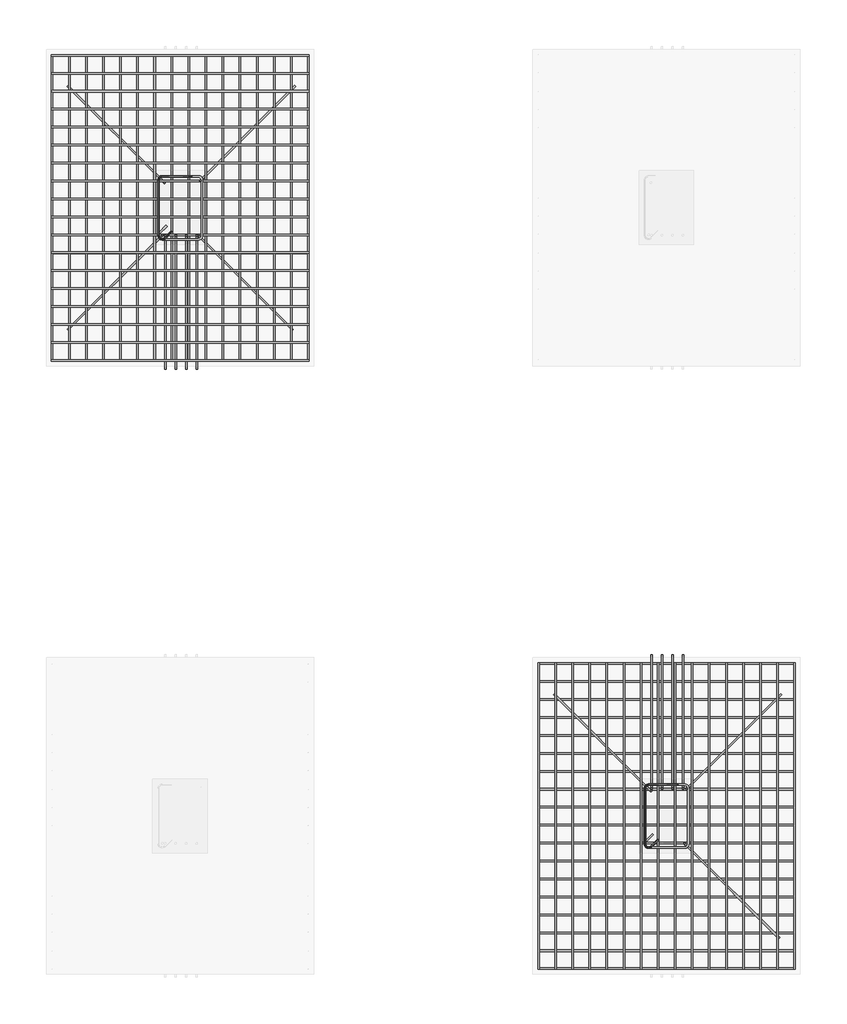
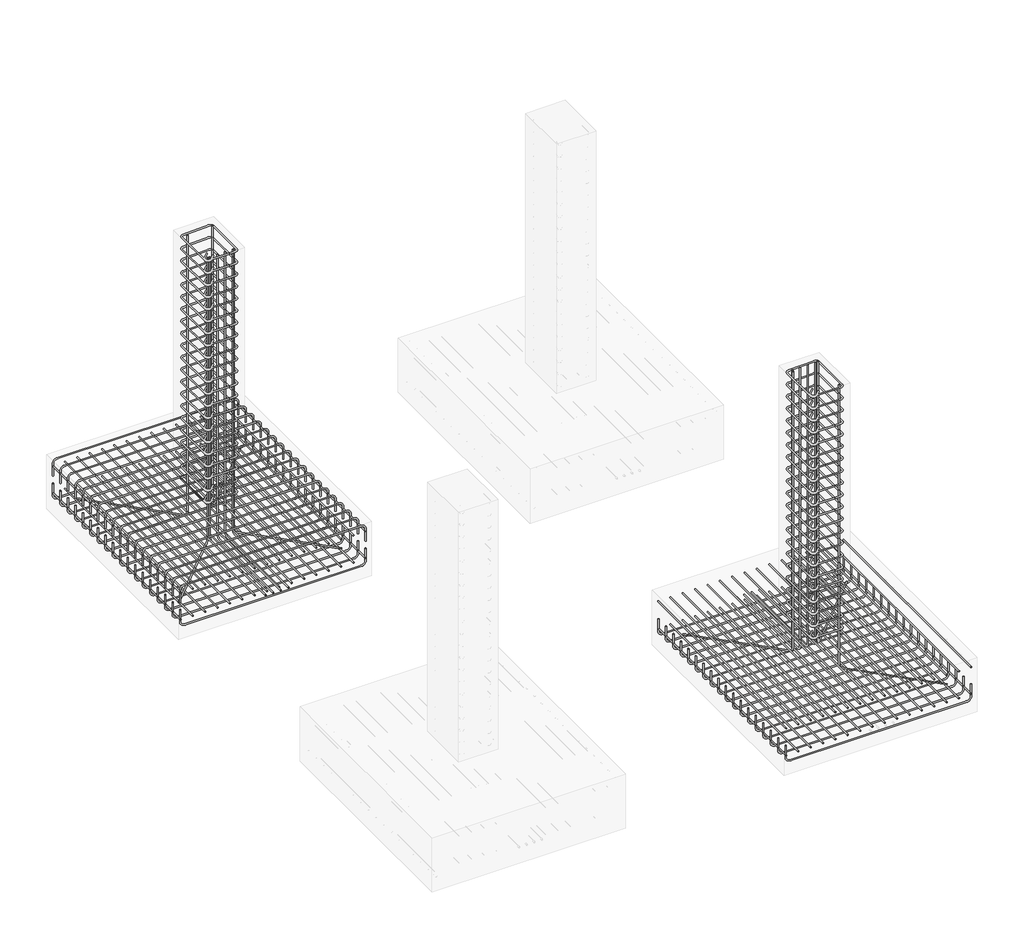
# One storey, part 14 of 33: 18 reinforcing bars.
"""IFC4 building model written with IfcOpenShell, lengths in millimetres."""

from ifc_helpers import new_model, si_unit, point, frame, origin, place, context, project, spatial, polyline, circle_curve, trimmed, segment, composite_curve, source, transform, mapped, element, save
from ifc_brep_helpers import swept_disk

model = new_model("IFC4")

# Units and contexts
model_context = context("Model", 3, world=origin())
ifc_project = project(units=[si_unit("LENGTHUNIT", "METRE", prefix="MILLI")], contexts=[model_context])

# Site, building, storey
site = spatial("IfcSite", under=ifc_project)
building = spatial("IfcBuilding", under=site)
storey = spatial("IfcBuildingStorey", under=building, Elevation=-3000.0)

# Reinforcing bars
placement = place(None, origin())
reinforcing_bar_shape = source(origin(), model_context, "Body", "SolidModel", [
    swept_disk(composite_curve([segment(polyline([(-8586.1642742, 2955.9391866, -3330.080452), (-8586.1642742, 2955.9391866, -3477.380452)]), True, "CONTINUOUS"), segment(trimmed(circle_curve(frame((-8632.5142742, 2955.9391866, -3477.380452), z_axis=(0.0, 1.0, 0.0), x_axis=(46.350000000000364, 0.0, 0.0)), 46.35), [point((-8586.1642742, 2955.9391866, -3477.380452))], [point((-8632.5142742, 2955.9391866, -3523.730452))], True, "CARTESIAN"), True, "CONTINUOUS"), segment(polyline([(-8632.5142742, 2955.9391866, -3523.730452), (-10647.1142742, 2955.9391866, -3523.730452)]), True, "CONTINUOUS"), segment(trimmed(circle_curve(frame((-10647.1142742, 2955.9391866, -3477.380452), z_axis=(0.0, 1.0, 0.0), x_axis=(0.0, 0.0, -46.34999999999991)), 46.35), [point((-10647.1142742, 2955.9391866, -3523.730452))], [point((-10693.4642742, 2955.9391866, -3477.380452))], True, "CARTESIAN"), True, "CONTINUOUS"), segment(polyline([(-10693.4642742, 2955.9391866, -3477.380452), (-10693.4642742, 2955.9391866, -3330.080452)]), True, "CONTINUOUS")], self_intersect=False), 6.35),
])
element("IfcReinforcingBar", 1, at=placement, inside=storey, context=model_context, shape_type="MappedRepresentation", body=[
    mapped(reinforcing_bar_shape, transform((0.0, 0.0, 0.0), x_axis=(1.0, 0.0, 0.0), y_axis=(0.0, 1.0, 0.0), z_axis=(0.0, 0.0, 1.0))),
    mapped(reinforcing_bar_shape, transform((0.0, -147.4882353, 0.0), x_axis=(1.0, 0.0, 0.0), y_axis=(0.0, 1.0, 0.0), z_axis=(0.0, 0.0, 1.0))),
    mapped(reinforcing_bar_shape, transform((0.0, -294.9764706, 0.0), x_axis=(1.0, 0.0, 0.0), y_axis=(0.0, 1.0, 0.0), z_axis=(0.0, 0.0, 1.0))),
    mapped(reinforcing_bar_shape, transform((0.0, -442.4647059, 0.0), x_axis=(1.0, 0.0, 0.0), y_axis=(0.0, 1.0, 0.0), z_axis=(0.0, 0.0, 1.0))),
    mapped(reinforcing_bar_shape, transform((0.0, -589.9529412, 0.0), x_axis=(1.0, 0.0, 0.0), y_axis=(0.0, 1.0, 0.0), z_axis=(0.0, 0.0, 1.0))),
    mapped(reinforcing_bar_shape, transform((0.0, -737.4411765, 0.0), x_axis=(1.0, 0.0, 0.0), y_axis=(0.0, 1.0, 0.0), z_axis=(0.0, 0.0, 1.0))),
    mapped(reinforcing_bar_shape, transform((0.0, -884.9294118, 0.0), x_axis=(1.0, 0.0, 0.0), y_axis=(0.0, 1.0, 0.0), z_axis=(0.0, 0.0, 1.0))),
    mapped(reinforcing_bar_shape, transform((0.0, -1032.4176471, 0.0), x_axis=(1.0, 0.0, 0.0), y_axis=(0.0, 1.0, 0.0), z_axis=(0.0, 0.0, 1.0))),
    mapped(reinforcing_bar_shape, transform((0.0, -1179.9058824, 0.0), x_axis=(1.0, 0.0, 0.0), y_axis=(0.0, 1.0, 0.0), z_axis=(0.0, 0.0, 1.0))),
    mapped(reinforcing_bar_shape, transform((0.0, -1327.3941176, 0.0), x_axis=(1.0, 0.0, 0.0), y_axis=(0.0, 1.0, 0.0), z_axis=(0.0, 0.0, 1.0))),
    mapped(reinforcing_bar_shape, transform((0.0, -1474.8823529, 0.0), x_axis=(1.0, 0.0, 0.0), y_axis=(0.0, 1.0, 0.0), z_axis=(0.0, 0.0, 1.0))),
    mapped(reinforcing_bar_shape, transform((0.0, -1622.3705882, 0.0), x_axis=(1.0, 0.0, 0.0), y_axis=(0.0, 1.0, 0.0), z_axis=(0.0, 0.0, 1.0))),
    mapped(reinforcing_bar_shape, transform((0.0, -1769.8588235, 0.0), x_axis=(1.0, 0.0, 0.0), y_axis=(0.0, 1.0, 0.0), z_axis=(0.0, 0.0, 1.0))),
    mapped(reinforcing_bar_shape, transform((0.0, -1917.3470588, 0.0), x_axis=(1.0, 0.0, 0.0), y_axis=(0.0, 1.0, 0.0), z_axis=(0.0, 0.0, 1.0))),
    mapped(reinforcing_bar_shape, transform((0.0, -2064.8352941, 0.0), x_axis=(1.0, 0.0, 0.0), y_axis=(0.0, 1.0, 0.0), z_axis=(0.0, 0.0, 1.0))),
    mapped(reinforcing_bar_shape, transform((0.0, -2212.3235294, 0.0), x_axis=(1.0, 0.0, 0.0), y_axis=(0.0, 1.0, 0.0), z_axis=(0.0, 0.0, 1.0))),
    mapped(reinforcing_bar_shape, transform((0.0, -2359.8117647, 0.0), x_axis=(1.0, 0.0, 0.0), y_axis=(0.0, 1.0, 0.0), z_axis=(0.0, 0.0, 1.0))),
    mapped(reinforcing_bar_shape, transform((0.0, -2507.3, 0.0), x_axis=(1.0, 0.0, 0.0), y_axis=(0.0, 1.0, 0.0), z_axis=(0.0, 0.0, 1.0))),
])
reinforcing_bar_2_shape = source(origin(), model_context, "Body", "SolidModel", [
    swept_disk(composite_curve([segment(polyline([(-8586.1642742, 442.2891866, -3447.8614173), (-8586.1642742, 2962.2891866, -3447.8614173)]), True, "CONTINUOUS")], self_intersect=False), 6.35),
])
element("IfcReinforcingBar", 2, at=placement, inside=storey, context=model_context, shape_type="MappedRepresentation", body=[
    mapped(reinforcing_bar_2_shape, transform((0.0, 0.0, 0.0), x_axis=(1.0, 0.0, 0.0), y_axis=(0.0, 1.0, 0.0), z_axis=(0.0, 0.0, 1.0))),
    mapped(reinforcing_bar_2_shape, transform((-140.4866667, 0.0, 0.0), x_axis=(1.0, 0.0, 0.0), y_axis=(0.0, 1.0, 0.0), z_axis=(0.0, 0.0, 1.0))),
    mapped(reinforcing_bar_2_shape, transform((-280.9733333, 0.0, 0.0), x_axis=(1.0, 0.0, 0.0), y_axis=(0.0, 1.0, 0.0), z_axis=(0.0, 0.0, 1.0))),
    mapped(reinforcing_bar_2_shape, transform((-421.46, 0.0, 0.0), x_axis=(1.0, 0.0, 0.0), y_axis=(0.0, 1.0, 0.0), z_axis=(0.0, 0.0, 1.0))),
    mapped(reinforcing_bar_2_shape, transform((-561.9466667, 0.0, 0.0), x_axis=(1.0, 0.0, 0.0), y_axis=(0.0, 1.0, 0.0), z_axis=(0.0, 0.0, 1.0))),
    mapped(reinforcing_bar_2_shape, transform((-702.4333333, 0.0, 0.0), x_axis=(1.0, 0.0, 0.0), y_axis=(0.0, 1.0, 0.0), z_axis=(0.0, 0.0, 1.0))),
    mapped(reinforcing_bar_2_shape, transform((-842.92, 0.0, 0.0), x_axis=(1.0, 0.0, 0.0), y_axis=(0.0, 1.0, 0.0), z_axis=(0.0, 0.0, 1.0))),
    mapped(reinforcing_bar_2_shape, transform((-983.4066667, 0.0, 0.0), x_axis=(1.0, 0.0, 0.0), y_axis=(0.0, 1.0, 0.0), z_axis=(0.0, 0.0, 1.0))),
    mapped(reinforcing_bar_2_shape, transform((-1123.8933333, 0.0, 0.0), x_axis=(1.0, 0.0, 0.0), y_axis=(0.0, 1.0, 0.0), z_axis=(0.0, 0.0, 1.0))),
    mapped(reinforcing_bar_2_shape, transform((-1264.38, 0.0, 0.0), x_axis=(1.0, 0.0, 0.0), y_axis=(0.0, 1.0, 0.0), z_axis=(0.0, 0.0, 1.0))),
    mapped(reinforcing_bar_2_shape, transform((-1404.8666667, 0.0, 0.0), x_axis=(1.0, 0.0, 0.0), y_axis=(0.0, 1.0, 0.0), z_axis=(0.0, 0.0, 1.0))),
    mapped(reinforcing_bar_2_shape, transform((-1545.3533333, 0.0, 0.0), x_axis=(1.0, 0.0, 0.0), y_axis=(0.0, 1.0, 0.0), z_axis=(0.0, 0.0, 1.0))),
    mapped(reinforcing_bar_2_shape, transform((-1685.84, 0.0, 0.0), x_axis=(1.0, 0.0, 0.0), y_axis=(0.0, 1.0, 0.0), z_axis=(0.0, 0.0, 1.0))),
    mapped(reinforcing_bar_2_shape, transform((-1826.3266667, 0.0, 0.0), x_axis=(1.0, 0.0, 0.0), y_axis=(0.0, 1.0, 0.0), z_axis=(0.0, 0.0, 1.0))),
    mapped(reinforcing_bar_2_shape, transform((-1966.8133333, 0.0, 0.0), x_axis=(1.0, 0.0, 0.0), y_axis=(0.0, 1.0, 0.0), z_axis=(0.0, 0.0, 1.0))),
    mapped(reinforcing_bar_2_shape, transform((-2107.3, 0.0, 0.0), x_axis=(1.0, 0.0, 0.0), y_axis=(0.0, 1.0, 0.0), z_axis=(0.0, 0.0, 1.0))),
])
reinforcing_bar_3_shape = source(origin(), model_context, "Body", "SolidModel", [
    swept_disk(composite_curve([segment(polyline([(-10693.4642742, 442.2891866, -3122.7084113), (-10693.4642742, 2962.2891866, -3122.7084113)]), True, "CONTINUOUS")], self_intersect=False), 6.35),
])
element("IfcReinforcingBar", 3, at=placement, inside=storey, context=model_context, shape_type="MappedRepresentation", body=[
    mapped(reinforcing_bar_3_shape, transform((0.0, 0.0, 0.0), x_axis=(1.0, 0.0, 0.0), y_axis=(0.0, 1.0, 0.0), z_axis=(0.0, 0.0, 1.0))),
    mapped(reinforcing_bar_3_shape, transform((140.4866667, 0.0, 0.0), x_axis=(1.0, 0.0, 0.0), y_axis=(0.0, 1.0, 0.0), z_axis=(0.0, 0.0, 1.0))),
    mapped(reinforcing_bar_3_shape, transform((280.9733333, 0.0, 0.0), x_axis=(1.0, 0.0, 0.0), y_axis=(0.0, 1.0, 0.0), z_axis=(0.0, 0.0, 1.0))),
    mapped(reinforcing_bar_3_shape, transform((421.46, 0.0, 0.0), x_axis=(1.0, 0.0, 0.0), y_axis=(0.0, 1.0, 0.0), z_axis=(0.0, 0.0, 1.0))),
    mapped(reinforcing_bar_3_shape, transform((561.9466667, 0.0, 0.0), x_axis=(1.0, 0.0, 0.0), y_axis=(0.0, 1.0, 0.0), z_axis=(0.0, 0.0, 1.0))),
    mapped(reinforcing_bar_3_shape, transform((702.4333333, 0.0, 0.0), x_axis=(1.0, 0.0, 0.0), y_axis=(0.0, 1.0, 0.0), z_axis=(0.0, 0.0, 1.0))),
    mapped(reinforcing_bar_3_shape, transform((842.92, 0.0, 0.0), x_axis=(1.0, 0.0, 0.0), y_axis=(0.0, 1.0, 0.0), z_axis=(0.0, 0.0, 1.0))),
    mapped(reinforcing_bar_3_shape, transform((983.4066667, 0.0, 0.0), x_axis=(1.0, 0.0, 0.0), y_axis=(0.0, 1.0, 0.0), z_axis=(0.0, 0.0, 1.0))),
    mapped(reinforcing_bar_3_shape, transform((1123.8933333, 0.0, 0.0), x_axis=(1.0, 0.0, 0.0), y_axis=(0.0, 1.0, 0.0), z_axis=(0.0, 0.0, 1.0))),
    mapped(reinforcing_bar_3_shape, transform((1264.38, 0.0, 0.0), x_axis=(1.0, 0.0, 0.0), y_axis=(0.0, 1.0, 0.0), z_axis=(0.0, 0.0, 1.0))),
    mapped(reinforcing_bar_3_shape, transform((1404.8666667, 0.0, 0.0), x_axis=(1.0, 0.0, 0.0), y_axis=(0.0, 1.0, 0.0), z_axis=(0.0, 0.0, 1.0))),
    mapped(reinforcing_bar_3_shape, transform((1545.3533333, 0.0, 0.0), x_axis=(1.0, 0.0, 0.0), y_axis=(0.0, 1.0, 0.0), z_axis=(0.0, 0.0, 1.0))),
    mapped(reinforcing_bar_3_shape, transform((1685.84, 0.0, 0.0), x_axis=(1.0, 0.0, 0.0), y_axis=(0.0, 1.0, 0.0), z_axis=(0.0, 0.0, 1.0))),
    mapped(reinforcing_bar_3_shape, transform((1826.3266667, 0.0, 0.0), x_axis=(1.0, 0.0, 0.0), y_axis=(0.0, 1.0, 0.0), z_axis=(0.0, 0.0, 1.0))),
    mapped(reinforcing_bar_3_shape, transform((1966.8133333, 0.0, 0.0), x_axis=(1.0, 0.0, 0.0), y_axis=(0.0, 1.0, 0.0), z_axis=(0.0, 0.0, 1.0))),
    mapped(reinforcing_bar_3_shape, transform((2107.3, 0.0, 0.0), x_axis=(1.0, 0.0, 0.0), y_axis=(0.0, 1.0, 0.0), z_axis=(0.0, 0.0, 1.0))),
])
reinforcing_bar_4_shape = source(origin(), model_context, "Body", "SolidModel", [
    swept_disk(composite_curve([segment(polyline([(-14693.4642742, 7955.9391866, -3240.0), (-14693.4642742, 7955.9391866, -3092.7)]), True, "CONTINUOUS"), segment(trimmed(circle_curve(frame((-14647.1142742, 7955.9391866, -3092.7), z_axis=(0.0, 1.0, 0.0), x_axis=(-46.350000000000364, 0.0, 0.0)), 46.35), [point((-14693.4642742, 7955.9391866, -3092.7))], [point((-14647.1142742, 7955.9391866, -3046.35))], True, "CARTESIAN"), True, "CONTINUOUS"), segment(polyline([(-14647.1142742, 7955.9391866, -3046.35), (-12632.5142742, 7955.9391866, -3046.35)]), True, "CONTINUOUS"), segment(trimmed(circle_curve(frame((-12632.5142742, 7955.9391866, -3092.7), z_axis=(0.0, 1.0, 0.0), x_axis=(0.0, 0.0, 46.34999999999991)), 46.35), [point((-12632.5142742, 7955.9391866, -3046.35))], [point((-12586.1642742, 7955.9391866, -3092.7))], True, "CARTESIAN"), True, "CONTINUOUS"), segment(polyline([(-12586.1642742, 7955.9391866, -3092.7), (-12586.1642742, 7955.9391866, -3240.0)]), True, "CONTINUOUS")], self_intersect=False), 6.35),
])
element("IfcReinforcingBar", 4, at=placement, inside=storey, context=model_context, shape_type="MappedRepresentation", body=[
    mapped(reinforcing_bar_4_shape, transform((0.0, 0.0, 0.0), x_axis=(1.0, 0.0, 0.0), y_axis=(0.0, 1.0, 0.0), z_axis=(0.0, 0.0, 1.0))),
    mapped(reinforcing_bar_4_shape, transform((0.0, -147.4882353, 0.0), x_axis=(1.0, 0.0, 0.0), y_axis=(0.0, 1.0, 0.0), z_axis=(0.0, 0.0, 1.0))),
    mapped(reinforcing_bar_4_shape, transform((0.0, -294.9764706, 0.0), x_axis=(1.0, 0.0, 0.0), y_axis=(0.0, 1.0, 0.0), z_axis=(0.0, 0.0, 1.0))),
    mapped(reinforcing_bar_4_shape, transform((0.0, -442.4647059, 0.0), x_axis=(1.0, 0.0, 0.0), y_axis=(0.0, 1.0, 0.0), z_axis=(0.0, 0.0, 1.0))),
    mapped(reinforcing_bar_4_shape, transform((0.0, -589.9529412, 0.0), x_axis=(1.0, 0.0, 0.0), y_axis=(0.0, 1.0, 0.0), z_axis=(0.0, 0.0, 1.0))),
    mapped(reinforcing_bar_4_shape, transform((0.0, -737.4411765, 0.0), x_axis=(1.0, 0.0, 0.0), y_axis=(0.0, 1.0, 0.0), z_axis=(0.0, 0.0, 1.0))),
    mapped(reinforcing_bar_4_shape, transform((0.0, -884.9294118, 0.0), x_axis=(1.0, 0.0, 0.0), y_axis=(0.0, 1.0, 0.0), z_axis=(0.0, 0.0, 1.0))),
    mapped(reinforcing_bar_4_shape, transform((0.0, -1032.4176471, 0.0), x_axis=(1.0, 0.0, 0.0), y_axis=(0.0, 1.0, 0.0), z_axis=(0.0, 0.0, 1.0))),
    mapped(reinforcing_bar_4_shape, transform((0.0, -1179.9058824, 0.0), x_axis=(1.0, 0.0, 0.0), y_axis=(0.0, 1.0, 0.0), z_axis=(0.0, 0.0, 1.0))),
    mapped(reinforcing_bar_4_shape, transform((0.0, -1327.3941176, 0.0), x_axis=(1.0, 0.0, 0.0), y_axis=(0.0, 1.0, 0.0), z_axis=(0.0, 0.0, 1.0))),
    mapped(reinforcing_bar_4_shape, transform((0.0, -1474.8823529, 0.0), x_axis=(1.0, 0.0, 0.0), y_axis=(0.0, 1.0, 0.0), z_axis=(0.0, 0.0, 1.0))),
    mapped(reinforcing_bar_4_shape, transform((0.0, -1622.3705882, 0.0), x_axis=(1.0, 0.0, 0.0), y_axis=(0.0, 1.0, 0.0), z_axis=(0.0, 0.0, 1.0))),
    mapped(reinforcing_bar_4_shape, transform((0.0, -1769.8588235, 0.0), x_axis=(1.0, 0.0, 0.0), y_axis=(0.0, 1.0, 0.0), z_axis=(0.0, 0.0, 1.0))),
    mapped(reinforcing_bar_4_shape, transform((0.0, -1917.3470588, 0.0), x_axis=(1.0, 0.0, 0.0), y_axis=(0.0, 1.0, 0.0), z_axis=(0.0, 0.0, 1.0))),
    mapped(reinforcing_bar_4_shape, transform((0.0, -2064.8352941, 0.0), x_axis=(1.0, 0.0, 0.0), y_axis=(0.0, 1.0, 0.0), z_axis=(0.0, 0.0, 1.0))),
    mapped(reinforcing_bar_4_shape, transform((0.0, -2212.3235294, 0.0), x_axis=(1.0, 0.0, 0.0), y_axis=(0.0, 1.0, 0.0), z_axis=(0.0, 0.0, 1.0))),
    mapped(reinforcing_bar_4_shape, transform((0.0, -2359.8117647, 0.0), x_axis=(1.0, 0.0, 0.0), y_axis=(0.0, 1.0, 0.0), z_axis=(0.0, 0.0, 1.0))),
    mapped(reinforcing_bar_4_shape, transform((0.0, -2507.3, 0.0), x_axis=(1.0, 0.0, 0.0), y_axis=(0.0, 1.0, 0.0), z_axis=(0.0, 0.0, 1.0))),
])
reinforcing_bar_5_shape = source(origin(), model_context, "Body", "SolidModel", [
    swept_disk(composite_curve([segment(polyline([(-12586.1642742, 7955.9391866, -3330.080452), (-12586.1642742, 7955.9391866, -3477.380452)]), True, "CONTINUOUS"), segment(trimmed(circle_curve(frame((-12632.5142742, 7955.9391866, -3477.380452), z_axis=(0.0, 1.0, 0.0), x_axis=(46.350000000000364, 0.0, 0.0)), 46.35), [point((-12586.1642742, 7955.9391866, -3477.380452))], [point((-12632.5142742, 7955.9391866, -3523.730452))], True, "CARTESIAN"), True, "CONTINUOUS"), segment(polyline([(-12632.5142742, 7955.9391866, -3523.730452), (-14647.1142742, 7955.9391866, -3523.730452)]), True, "CONTINUOUS"), segment(trimmed(circle_curve(frame((-14647.1142742, 7955.9391866, -3477.380452), z_axis=(0.0, 1.0, 0.0), x_axis=(0.0, 0.0, -46.34999999999991)), 46.35), [point((-14647.1142742, 7955.9391866, -3523.730452))], [point((-14693.4642742, 7955.9391866, -3477.380452))], True, "CARTESIAN"), True, "CONTINUOUS"), segment(polyline([(-14693.4642742, 7955.9391866, -3477.380452), (-14693.4642742, 7955.9391866, -3330.080452)]), True, "CONTINUOUS")], self_intersect=False), 6.35),
])
element("IfcReinforcingBar", 5, at=placement, inside=storey, context=model_context, shape_type="MappedRepresentation", body=[
    mapped(reinforcing_bar_5_shape, transform((0.0, 0.0, 0.0), x_axis=(1.0, 0.0, 0.0), y_axis=(0.0, 1.0, 0.0), z_axis=(0.0, 0.0, 1.0))),
    mapped(reinforcing_bar_5_shape, transform((0.0, -147.4882353, 0.0), x_axis=(1.0, 0.0, 0.0), y_axis=(0.0, 1.0, 0.0), z_axis=(0.0, 0.0, 1.0))),
    mapped(reinforcing_bar_5_shape, transform((0.0, -294.9764706, 0.0), x_axis=(1.0, 0.0, 0.0), y_axis=(0.0, 1.0, 0.0), z_axis=(0.0, 0.0, 1.0))),
    mapped(reinforcing_bar_5_shape, transform((0.0, -442.4647059, 0.0), x_axis=(1.0, 0.0, 0.0), y_axis=(0.0, 1.0, 0.0), z_axis=(0.0, 0.0, 1.0))),
    mapped(reinforcing_bar_5_shape, transform((0.0, -589.9529412, 0.0), x_axis=(1.0, 0.0, 0.0), y_axis=(0.0, 1.0, 0.0), z_axis=(0.0, 0.0, 1.0))),
    mapped(reinforcing_bar_5_shape, transform((0.0, -737.4411765, 0.0), x_axis=(1.0, 0.0, 0.0), y_axis=(0.0, 1.0, 0.0), z_axis=(0.0, 0.0, 1.0))),
    mapped(reinforcing_bar_5_shape, transform((0.0, -884.9294118, 0.0), x_axis=(1.0, 0.0, 0.0), y_axis=(0.0, 1.0, 0.0), z_axis=(0.0, 0.0, 1.0))),
    mapped(reinforcing_bar_5_shape, transform((0.0, -1032.4176471, 0.0), x_axis=(1.0, 0.0, 0.0), y_axis=(0.0, 1.0, 0.0), z_axis=(0.0, 0.0, 1.0))),
    mapped(reinforcing_bar_5_shape, transform((0.0, -1179.9058824, 0.0), x_axis=(1.0, 0.0, 0.0), y_axis=(0.0, 1.0, 0.0), z_axis=(0.0, 0.0, 1.0))),
    mapped(reinforcing_bar_5_shape, transform((0.0, -1327.3941176, 0.0), x_axis=(1.0, 0.0, 0.0), y_axis=(0.0, 1.0, 0.0), z_axis=(0.0, 0.0, 1.0))),
    mapped(reinforcing_bar_5_shape, transform((0.0, -1474.8823529, 0.0), x_axis=(1.0, 0.0, 0.0), y_axis=(0.0, 1.0, 0.0), z_axis=(0.0, 0.0, 1.0))),
    mapped(reinforcing_bar_5_shape, transform((0.0, -1622.3705882, 0.0), x_axis=(1.0, 0.0, 0.0), y_axis=(0.0, 1.0, 0.0), z_axis=(0.0, 0.0, 1.0))),
    mapped(reinforcing_bar_5_shape, transform((0.0, -1769.8588235, 0.0), x_axis=(1.0, 0.0, 0.0), y_axis=(0.0, 1.0, 0.0), z_axis=(0.0, 0.0, 1.0))),
    mapped(reinforcing_bar_5_shape, transform((0.0, -1917.3470588, 0.0), x_axis=(1.0, 0.0, 0.0), y_axis=(0.0, 1.0, 0.0), z_axis=(0.0, 0.0, 1.0))),
    mapped(reinforcing_bar_5_shape, transform((0.0, -2064.8352941, 0.0), x_axis=(1.0, 0.0, 0.0), y_axis=(0.0, 1.0, 0.0), z_axis=(0.0, 0.0, 1.0))),
    mapped(reinforcing_bar_5_shape, transform((0.0, -2212.3235294, 0.0), x_axis=(1.0, 0.0, 0.0), y_axis=(0.0, 1.0, 0.0), z_axis=(0.0, 0.0, 1.0))),
    mapped(reinforcing_bar_5_shape, transform((0.0, -2359.8117647, 0.0), x_axis=(1.0, 0.0, 0.0), y_axis=(0.0, 1.0, 0.0), z_axis=(0.0, 0.0, 1.0))),
    mapped(reinforcing_bar_5_shape, transform((0.0, -2507.3, 0.0), x_axis=(1.0, 0.0, 0.0), y_axis=(0.0, 1.0, 0.0), z_axis=(0.0, 0.0, 1.0))),
])
reinforcing_bar_6_shape = source(origin(), model_context, "Body", "SolidModel", [
    swept_disk(composite_curve([segment(polyline([(-12586.1642742, 5442.2891866, -3447.8614173), (-12586.1642742, 7962.2891866, -3447.8614173)]), True, "CONTINUOUS")], self_intersect=False), 6.35),
])
element("IfcReinforcingBar", 6, at=placement, inside=storey, context=model_context, shape_type="MappedRepresentation", body=[
    mapped(reinforcing_bar_6_shape, transform((0.0, 0.0, 0.0), x_axis=(1.0, 0.0, 0.0), y_axis=(0.0, 1.0, 0.0), z_axis=(0.0, 0.0, 1.0))),
    mapped(reinforcing_bar_6_shape, transform((-140.4866667, 0.0, 0.0), x_axis=(1.0, 0.0, 0.0), y_axis=(0.0, 1.0, 0.0), z_axis=(0.0, 0.0, 1.0))),
    mapped(reinforcing_bar_6_shape, transform((-280.9733333, 0.0, 0.0), x_axis=(1.0, 0.0, 0.0), y_axis=(0.0, 1.0, 0.0), z_axis=(0.0, 0.0, 1.0))),
    mapped(reinforcing_bar_6_shape, transform((-421.46, 0.0, 0.0), x_axis=(1.0, 0.0, 0.0), y_axis=(0.0, 1.0, 0.0), z_axis=(0.0, 0.0, 1.0))),
    mapped(reinforcing_bar_6_shape, transform((-561.9466667, 0.0, 0.0), x_axis=(1.0, 0.0, 0.0), y_axis=(0.0, 1.0, 0.0), z_axis=(0.0, 0.0, 1.0))),
    mapped(reinforcing_bar_6_shape, transform((-702.4333333, 0.0, 0.0), x_axis=(1.0, 0.0, 0.0), y_axis=(0.0, 1.0, 0.0), z_axis=(0.0, 0.0, 1.0))),
    mapped(reinforcing_bar_6_shape, transform((-842.92, 0.0, 0.0), x_axis=(1.0, 0.0, 0.0), y_axis=(0.0, 1.0, 0.0), z_axis=(0.0, 0.0, 1.0))),
    mapped(reinforcing_bar_6_shape, transform((-983.4066667, 0.0, 0.0), x_axis=(1.0, 0.0, 0.0), y_axis=(0.0, 1.0, 0.0), z_axis=(0.0, 0.0, 1.0))),
    mapped(reinforcing_bar_6_shape, transform((-1123.8933333, 0.0, 0.0), x_axis=(1.0, 0.0, 0.0), y_axis=(0.0, 1.0, 0.0), z_axis=(0.0, 0.0, 1.0))),
    mapped(reinforcing_bar_6_shape, transform((-1264.38, 0.0, 0.0), x_axis=(1.0, 0.0, 0.0), y_axis=(0.0, 1.0, 0.0), z_axis=(0.0, 0.0, 1.0))),
    mapped(reinforcing_bar_6_shape, transform((-1404.8666667, 0.0, 0.0), x_axis=(1.0, 0.0, 0.0), y_axis=(0.0, 1.0, 0.0), z_axis=(0.0, 0.0, 1.0))),
    mapped(reinforcing_bar_6_shape, transform((-1545.3533333, 0.0, 0.0), x_axis=(1.0, 0.0, 0.0), y_axis=(0.0, 1.0, 0.0), z_axis=(0.0, 0.0, 1.0))),
    mapped(reinforcing_bar_6_shape, transform((-1685.84, 0.0, 0.0), x_axis=(1.0, 0.0, 0.0), y_axis=(0.0, 1.0, 0.0), z_axis=(0.0, 0.0, 1.0))),
    mapped(reinforcing_bar_6_shape, transform((-1826.3266667, 0.0, 0.0), x_axis=(1.0, 0.0, 0.0), y_axis=(0.0, 1.0, 0.0), z_axis=(0.0, 0.0, 1.0))),
    mapped(reinforcing_bar_6_shape, transform((-1966.8133333, 0.0, 0.0), x_axis=(1.0, 0.0, 0.0), y_axis=(0.0, 1.0, 0.0), z_axis=(0.0, 0.0, 1.0))),
    mapped(reinforcing_bar_6_shape, transform((-2107.3, 0.0, 0.0), x_axis=(1.0, 0.0, 0.0), y_axis=(0.0, 1.0, 0.0), z_axis=(0.0, 0.0, 1.0))),
])
reinforcing_bar_7_shape = source(origin(), model_context, "Body", "SolidModel", [
    swept_disk(composite_curve([segment(polyline([(-14693.4642742, 5442.2891866, -3122.7084113), (-14693.4642742, 7962.2891866, -3122.7084113)]), True, "CONTINUOUS")], self_intersect=False), 6.35),
])
element("IfcReinforcingBar", 7, at=placement, inside=storey, context=model_context, shape_type="MappedRepresentation", body=[
    mapped(reinforcing_bar_7_shape, transform((0.0, 0.0, 0.0), x_axis=(1.0, 0.0, 0.0), y_axis=(0.0, 1.0, 0.0), z_axis=(0.0, 0.0, 1.0))),
    mapped(reinforcing_bar_7_shape, transform((140.4866667, 0.0, 0.0), x_axis=(1.0, 0.0, 0.0), y_axis=(0.0, 1.0, 0.0), z_axis=(0.0, 0.0, 1.0))),
    mapped(reinforcing_bar_7_shape, transform((280.9733333, 0.0, 0.0), x_axis=(1.0, 0.0, 0.0), y_axis=(0.0, 1.0, 0.0), z_axis=(0.0, 0.0, 1.0))),
    mapped(reinforcing_bar_7_shape, transform((421.46, 0.0, 0.0), x_axis=(1.0, 0.0, 0.0), y_axis=(0.0, 1.0, 0.0), z_axis=(0.0, 0.0, 1.0))),
    mapped(reinforcing_bar_7_shape, transform((561.9466667, 0.0, 0.0), x_axis=(1.0, 0.0, 0.0), y_axis=(0.0, 1.0, 0.0), z_axis=(0.0, 0.0, 1.0))),
    mapped(reinforcing_bar_7_shape, transform((702.4333333, 0.0, 0.0), x_axis=(1.0, 0.0, 0.0), y_axis=(0.0, 1.0, 0.0), z_axis=(0.0, 0.0, 1.0))),
    mapped(reinforcing_bar_7_shape, transform((842.92, 0.0, 0.0), x_axis=(1.0, 0.0, 0.0), y_axis=(0.0, 1.0, 0.0), z_axis=(0.0, 0.0, 1.0))),
    mapped(reinforcing_bar_7_shape, transform((983.4066667, 0.0, 0.0), x_axis=(1.0, 0.0, 0.0), y_axis=(0.0, 1.0, 0.0), z_axis=(0.0, 0.0, 1.0))),
    mapped(reinforcing_bar_7_shape, transform((1123.8933333, 0.0, 0.0), x_axis=(1.0, 0.0, 0.0), y_axis=(0.0, 1.0, 0.0), z_axis=(0.0, 0.0, 1.0))),
    mapped(reinforcing_bar_7_shape, transform((1264.38, 0.0, 0.0), x_axis=(1.0, 0.0, 0.0), y_axis=(0.0, 1.0, 0.0), z_axis=(0.0, 0.0, 1.0))),
    mapped(reinforcing_bar_7_shape, transform((1404.8666667, 0.0, 0.0), x_axis=(1.0, 0.0, 0.0), y_axis=(0.0, 1.0, 0.0), z_axis=(0.0, 0.0, 1.0))),
    mapped(reinforcing_bar_7_shape, transform((1545.3533333, 0.0, 0.0), x_axis=(1.0, 0.0, 0.0), y_axis=(0.0, 1.0, 0.0), z_axis=(0.0, 0.0, 1.0))),
    mapped(reinforcing_bar_7_shape, transform((1685.84, 0.0, 0.0), x_axis=(1.0, 0.0, 0.0), y_axis=(0.0, 1.0, 0.0), z_axis=(0.0, 0.0, 1.0))),
    mapped(reinforcing_bar_7_shape, transform((1826.3266667, 0.0, 0.0), x_axis=(1.0, 0.0, 0.0), y_axis=(0.0, 1.0, 0.0), z_axis=(0.0, 0.0, 1.0))),
    mapped(reinforcing_bar_7_shape, transform((1966.8133333, 0.0, 0.0), x_axis=(1.0, 0.0, 0.0), y_axis=(0.0, 1.0, 0.0), z_axis=(0.0, 0.0, 1.0))),
    mapped(reinforcing_bar_7_shape, transform((2107.3, 0.0, 0.0), x_axis=(1.0, 0.0, 0.0), y_axis=(0.0, 1.0, 0.0), z_axis=(0.0, 0.0, 1.0))),
])
reinforcing_bar_8_shape = source(origin(), model_context, "Body", "SolidModel", [
    swept_disk(composite_curve([segment(polyline([(-13753.5385089, 6553.1005472, -2953.65), (-13809.2820718, 6497.3569842, -2953.65)]), True, "CONTINUOUS"), segment(trimmed(circle_curve(frame((-13787.1142742, 6475.1891866, -2953.65), z_axis=(0.0, 0.0, 1.0), x_axis=(-22.167797600000995, 22.167797600000085, 0.0)), 31.35), [point((-13809.2820718, 6497.3569842, -2953.65))], [point((-13787.1142742, 6443.8391866, -2953.65))], True, "CARTESIAN"), True, "CONTINUOUS"), segment(polyline([(-13787.1142742, 6443.8391866, -2953.65), (-13492.5142742, 6443.8391866, -2953.65)]), True, "CONTINUOUS"), segment(trimmed(circle_curve(frame((-13492.5142742, 6475.1891866, -2953.65), z_axis=(0.0, 0.0, 1.0), x_axis=(0.0, -31.349999999999454, 0.0)), 31.35), [point((-13492.5142742, 6443.8391866, -2953.65))], [point((-13461.1642742, 6475.1891866, -2953.65))], True, "CARTESIAN"), True, "CONTINUOUS"), segment(polyline([(-13461.1642742, 6475.1891866, -2953.65), (-13461.1642742, 6929.3891866, -2953.65)]), True, "CONTINUOUS"), segment(trimmed(circle_curve(frame((-13492.4944891, 6929.3891866, -2954.7636125), z_axis=(-0.0355219283344822, 0.0, 0.9993688971583016), x_axis=(31.33021489999919, 0.0, 1.1136124999998174)), 31.35), [point((-13461.1642742, 6929.3891866, -2953.65))], [point((-13492.4944891, 6960.7391866, -2954.7636125))], True, "CARTESIAN"), True, "CONTINUOUS"), segment(polyline([(-13492.4944891, 6960.7391866, -2954.7636125), (-13787.1340593, 6960.7391866, -2965.2363875)]), True, "CONTINUOUS"), segment(trimmed(circle_curve(frame((-13787.1340593, 6929.3891866, -2965.2363875), z_axis=(-0.0355219283344822, 0.0, 0.9993688971583016), x_axis=(0.0, 31.349999999999454, 0.0)), 31.35), [point((-13787.1340593, 6960.7391866, -2965.2363875))], [point((-13818.4642742, 6929.3891866, -2966.35))], True, "CARTESIAN"), True, "CONTINUOUS"), segment(polyline([(-13818.4642742, 6929.3891866, -2966.35), (-13818.4642742, 6475.1891866, -2966.35)]), True, "CONTINUOUS"), segment(trimmed(circle_curve(frame((-13787.1142742, 6475.1891866, -2966.35), z_axis=(0.0, 0.0, 1.0), x_axis=(-31.350000000000364, 0.0, 0.0)), 31.35), [point((-13818.4642742, 6475.1891866, -2966.35))], [point((-13764.9464766, 6453.021389, -2966.35))], True, "CARTESIAN"), True, "CONTINUOUS"), segment(polyline([(-13764.9464766, 6453.021389, -2966.35), (-13709.2029137, 6508.764952, -2966.35)]), True, "CONTINUOUS")], self_intersect=False), 6.35),
])
element("IfcReinforcingBar", 8, at=placement, inside=storey, context=model_context, shape_type="MappedRepresentation", body=[
    mapped(reinforcing_bar_8_shape, transform((0.0, 0.0, 0.0), x_axis=(1.0, 0.0, 0.0), y_axis=(0.0, 1.0, 0.0), z_axis=(0.0, 0.0, 1.0))),
    mapped(reinforcing_bar_8_shape, transform((0.0, 0.0, 145.365), x_axis=(1.0, 0.0, 0.0), y_axis=(0.0, 1.0, 0.0), z_axis=(0.0, 0.0, 1.0))),
    mapped(reinforcing_bar_8_shape, transform((0.0, 0.0, 290.73), x_axis=(1.0, 0.0, 0.0), y_axis=(0.0, 1.0, 0.0), z_axis=(0.0, 0.0, 1.0))),
    mapped(reinforcing_bar_8_shape, transform((0.0, 0.0, 436.095), x_axis=(1.0, 0.0, 0.0), y_axis=(0.0, 1.0, 0.0), z_axis=(0.0, 0.0, 1.0))),
    mapped(reinforcing_bar_8_shape, transform((0.0, 0.0, 581.46), x_axis=(1.0, 0.0, 0.0), y_axis=(0.0, 1.0, 0.0), z_axis=(0.0, 0.0, 1.0))),
    mapped(reinforcing_bar_8_shape, transform((0.0, 0.0, 726.825), x_axis=(1.0, 0.0, 0.0), y_axis=(0.0, 1.0, 0.0), z_axis=(0.0, 0.0, 1.0))),
    mapped(reinforcing_bar_8_shape, transform((0.0, 0.0, 872.19), x_axis=(1.0, 0.0, 0.0), y_axis=(0.0, 1.0, 0.0), z_axis=(0.0, 0.0, 1.0))),
    mapped(reinforcing_bar_8_shape, transform((0.0, 0.0, 1017.555), x_axis=(1.0, 0.0, 0.0), y_axis=(0.0, 1.0, 0.0), z_axis=(0.0, 0.0, 1.0))),
    mapped(reinforcing_bar_8_shape, transform((0.0, 0.0, 1162.92), x_axis=(1.0, 0.0, 0.0), y_axis=(0.0, 1.0, 0.0), z_axis=(0.0, 0.0, 1.0))),
    mapped(reinforcing_bar_8_shape, transform((0.0, 0.0, 1308.285), x_axis=(1.0, 0.0, 0.0), y_axis=(0.0, 1.0, 0.0), z_axis=(0.0, 0.0, 1.0))),
    mapped(reinforcing_bar_8_shape, transform((0.0, 0.0, 1453.65), x_axis=(1.0, 0.0, 0.0), y_axis=(0.0, 1.0, 0.0), z_axis=(0.0, 0.0, 1.0))),
    mapped(reinforcing_bar_8_shape, transform((0.0, 0.0, 1599.015), x_axis=(1.0, 0.0, 0.0), y_axis=(0.0, 1.0, 0.0), z_axis=(0.0, 0.0, 1.0))),
    mapped(reinforcing_bar_8_shape, transform((0.0, 0.0, 1744.38), x_axis=(1.0, 0.0, 0.0), y_axis=(0.0, 1.0, 0.0), z_axis=(0.0, 0.0, 1.0))),
    mapped(reinforcing_bar_8_shape, transform((0.0, 0.0, 1889.745), x_axis=(1.0, 0.0, 0.0), y_axis=(0.0, 1.0, 0.0), z_axis=(0.0, 0.0, 1.0))),
    mapped(reinforcing_bar_8_shape, transform((0.0, 0.0, 2035.11), x_axis=(1.0, 0.0, 0.0), y_axis=(0.0, 1.0, 0.0), z_axis=(0.0, 0.0, 1.0))),
    mapped(reinforcing_bar_8_shape, transform((0.0, 0.0, 2180.475), x_axis=(1.0, 0.0, 0.0), y_axis=(0.0, 1.0, 0.0), z_axis=(0.0, 0.0, 1.0))),
    mapped(reinforcing_bar_8_shape, transform((0.0, 0.0, 2325.84), x_axis=(1.0, 0.0, 0.0), y_axis=(0.0, 1.0, 0.0), z_axis=(0.0, 0.0, 1.0))),
    mapped(reinforcing_bar_8_shape, transform((0.0, 0.0, 2471.205), x_axis=(1.0, 0.0, 0.0), y_axis=(0.0, 1.0, 0.0), z_axis=(0.0, 0.0, 1.0))),
    mapped(reinforcing_bar_8_shape, transform((0.0, 0.0, 2616.57), x_axis=(1.0, 0.0, 0.0), y_axis=(0.0, 1.0, 0.0), z_axis=(0.0, 0.0, 1.0))),
    mapped(reinforcing_bar_8_shape, transform((0.0, 0.0, 2761.935), x_axis=(1.0, 0.0, 0.0), y_axis=(0.0, 1.0, 0.0), z_axis=(0.0, 0.0, 1.0))),
    mapped(reinforcing_bar_8_shape, transform((0.0, 0.0, 2907.3), x_axis=(1.0, 0.0, 0.0), y_axis=(0.0, 1.0, 0.0), z_axis=(0.0, 0.0, 1.0))),
])
element("IfcReinforcingBar", 9, at=placement, inside=storey, context=model_context, shape_type="SolidModel", body=[
    swept_disk(composite_curve([segment(polyline([(-13786.7956786, 6478.3660586, -40.0), (-13786.7956786, 6478.3660586, -3393.65)]), True, "CONTINUOUS"), segment(trimmed(circle_curve(frame((-13819.5700779, 6445.5916593, -3393.65), z_axis=(-0.7071067811865446, 0.7071067811865505, 0.0), x_axis=(32.77439930000037, 32.77439929999946, 0.0)), 46.35), [point((-13786.7956786, 6478.3660586, -3393.65))], [point((-13819.5700779, 6445.5916593, -3440.0))], True, "CARTESIAN"), True, "CONTINUOUS"), segment(polyline([(-13819.5700779, 6445.5916593, -3440.0), (-14564.6131379, 5700.5485993, -3440.0)]), True, "CONTINUOUS")], self_intersect=False), 6.35),
])
element("IfcReinforcingBar", 10, at=placement, inside=storey, context=model_context, shape_type="SolidModel", body=[
    swept_disk(composite_curve([segment(polyline([(-13768.8975726, 6908.3142087, -40.0), (-13768.8975726, 6908.3142087, -3361.434517)]), True, "CONTINUOUS"), segment(trimmed(circle_curve(frame((-13801.6719719, 6941.088608, -3361.434517), z_axis=(0.7071067811865539, 0.7071067811865411, 0.0), x_axis=(32.77439929999855, -32.77439930000037, 0.0)), 46.35), [point((-13768.8975726, 6908.3142087, -3361.434517))], [point((-13801.6719719, 6941.088608, -3407.784517))], True, "CARTESIAN"), True, "CONTINUOUS"), segment(polyline([(-13801.6719719, 6941.088608, -3407.784517), (-14564.6131379, 7704.029774, -3407.784517)]), True, "CONTINUOUS")], self_intersect=False), 6.35),
])
element("IfcReinforcingBar", 11, at=placement, inside=storey, context=model_context, shape_type="SolidModel", body=[
    swept_disk(composite_curve([segment(polyline([(-13492.8328699, 6478.3660586, -40.0), (-13492.8328699, 6478.3660586, -3393.65)]), True, "CONTINUOUS"), segment(trimmed(circle_curve(frame((-13460.0584706, 6445.5916593, -3393.65), z_axis=(-0.7071067811865493, -0.7071067811865459, 0.0), x_axis=(-32.77439929999855, 32.77439929999946, 0.0)), 46.35), [point((-13492.8328699, 6478.3660586, -3393.65))], [point((-13460.0584706, 6445.5916593, -3440.0))], True, "CARTESIAN"), True, "CONTINUOUS"), segment(polyline([(-13460.0584706, 6445.5916593, -3440.0), (-12715.0154106, 5700.5485993, -3440.0)]), True, "CONTINUOUS")], self_intersect=False), 6.35),
])
element("IfcReinforcingBar", 12, at=placement, inside=storey, context=model_context, shape_type="SolidModel", body=[
    swept_disk(composite_curve([segment(polyline([(-13474.2315783, 6926.2123147, -30.2564663), (-13474.2315783, 6926.2123147, -3383.9064663)]), True, "CONTINUOUS"), segment(trimmed(circle_curve(frame((-13441.457179, 6958.986714, -3383.9064663), z_axis=(0.7071067811865493, -0.7071067811865459, 0.0), x_axis=(-32.77439929999855, -32.77439929999946, 0.0)), 46.35), [point((-13474.2315783, 6926.2123147, -3383.9064663))], [point((-13441.457179, 6958.986714, -3430.2564663))], True, "CARTESIAN"), True, "CONTINUOUS"), segment(polyline([(-13441.457179, 6958.986714, -3430.2564663), (-12696.414119, 7704.029774, -3430.2564663)]), True, "CONTINUOUS")], self_intersect=False), 6.35),
])
reinforcing_bar_9_shape = source(origin(), model_context, "Body", "SolidModel", [
    swept_disk(composite_curve([segment(polyline([(-13763.8841678, 6476.5061866, -40.0), (-13763.8841678, 6476.5061866, -3393.65)]), True, "CONTINUOUS"), segment(trimmed(circle_curve(frame((-13763.8841678, 6430.1561866, -3393.65), z_axis=(-1.0, 0.0, 0.0), x_axis=(0.0, 46.349999999999454, 0.0)), 46.35), [point((-13763.8841678, 6476.5061866, -3393.65))], [point((-13763.8841678, 6430.1561866, -3440.0))], True, "CARTESIAN"), True, "CONTINUOUS"), segment(polyline([(-13763.8841678, 6430.1561866, -3440.0), (-13763.8841678, 5376.5061866, -3440.0)]), True, "CONTINUOUS")], self_intersect=False), 6.35),
])
element("IfcReinforcingBar", 13, at=placement, inside=storey, context=model_context, shape_type="MappedRepresentation", body=[
    mapped(reinforcing_bar_9_shape, transform((0.0, 0.0, 0.0), x_axis=(1.0, 0.0, 0.0), y_axis=(0.0, 1.0, 0.0), z_axis=(0.0, 0.0, 1.0))),
    mapped(reinforcing_bar_9_shape, transform((86.8979716, 0.0, 0.0), x_axis=(1.0, 0.0, 0.0), y_axis=(0.0, 1.0, 0.0), z_axis=(0.0, 0.0, 1.0))),
    mapped(reinforcing_bar_9_shape, transform((173.7959432, 0.0, 0.0), x_axis=(1.0, 0.0, 0.0), y_axis=(0.0, 1.0, 0.0), z_axis=(0.0, 0.0, 1.0))),
    mapped(reinforcing_bar_9_shape, transform((260.6939148, 0.0, 0.0), x_axis=(1.0, 0.0, 0.0), y_axis=(0.0, 1.0, 0.0), z_axis=(0.0, 0.0, 1.0))),
])
reinforcing_bar_10_shape = source(origin(), model_context, "Body", "SolidModel", [
    swept_disk(composite_curve([segment(polyline([(-9753.5385089, 1553.1005472, -2953.65), (-9809.2820718, 1497.3569842, -2953.65)]), True, "CONTINUOUS"), segment(trimmed(circle_curve(frame((-9787.1142742, 1475.1891866, -2953.65), z_axis=(0.0, 0.0, 1.0), x_axis=(-22.167797600000995, 22.167797599999858, 0.0)), 31.35), [point((-9809.2820718, 1497.3569842, -2953.65))], [point((-9787.1142742, 1443.8391866, -2953.65))], True, "CARTESIAN"), True, "CONTINUOUS"), segment(polyline([(-9787.1142742, 1443.8391866, -2953.65), (-9492.5142742, 1443.8391866, -2953.65)]), True, "CONTINUOUS"), segment(trimmed(circle_curve(frame((-9492.5142742, 1475.1891866, -2953.65), z_axis=(0.0, 0.0, 1.0), x_axis=(0.0, -31.350000000000136, 0.0)), 31.35), [point((-9492.5142742, 1443.8391866, -2953.65))], [point((-9461.1642742, 1475.1891866, -2953.65))], True, "CARTESIAN"), True, "CONTINUOUS"), segment(polyline([(-9461.1642742, 1475.1891866, -2953.65), (-9461.1642742, 1929.3891866, -2953.65)]), True, "CONTINUOUS"), segment(trimmed(circle_curve(frame((-9492.4944891, 1929.3891866, -2954.7636125), z_axis=(-0.0355219283344822, 0.0, 0.9993688971583016), x_axis=(31.33021489999919, 0.0, 1.1136124999998174)), 31.35), [point((-9461.1642742, 1929.3891866, -2953.65))], [point((-9492.4944891, 1960.7391866, -2954.7636125))], True, "CARTESIAN"), True, "CONTINUOUS"), segment(polyline([(-9492.4944891, 1960.7391866, -2954.7636125), (-9787.1340593, 1960.7391866, -2965.2363875)]), True, "CONTINUOUS"), segment(trimmed(circle_curve(frame((-9787.1340593, 1929.3891866, -2965.2363875), z_axis=(-0.0355219283344822, 0.0, 0.9993688971583016), x_axis=(0.0, 31.350000000000136, 0.0)), 31.35), [point((-9787.1340593, 1960.7391866, -2965.2363875))], [point((-9818.4642742, 1929.3891866, -2966.35))], True, "CARTESIAN"), True, "CONTINUOUS"), segment(polyline([(-9818.4642742, 1929.3891866, -2966.35), (-9818.4642742, 1475.1891866, -2966.35)]), True, "CONTINUOUS"), segment(trimmed(circle_curve(frame((-9787.1142742, 1475.1891866, -2966.35), z_axis=(0.0, 0.0, 1.0), x_axis=(-31.350000000000364, 0.0, 0.0)), 31.35), [point((-9818.4642742, 1475.1891866, -2966.35))], [point((-9764.9464766, 1453.021389, -2966.35))], True, "CARTESIAN"), True, "CONTINUOUS"), segment(polyline([(-9764.9464766, 1453.021389, -2966.35), (-9709.2029137, 1508.764952, -2966.35)]), True, "CONTINUOUS")], self_intersect=False), 6.35),
])
element("IfcReinforcingBar", 14, at=placement, inside=storey, context=model_context, shape_type="MappedRepresentation", body=[
    mapped(reinforcing_bar_10_shape, transform((0.0, 0.0, 0.0), x_axis=(1.0, 0.0, 0.0), y_axis=(0.0, 1.0, 0.0), z_axis=(0.0, 0.0, 1.0))),
    mapped(reinforcing_bar_10_shape, transform((0.0, 0.0, 145.365), x_axis=(1.0, 0.0, 0.0), y_axis=(0.0, 1.0, 0.0), z_axis=(0.0, 0.0, 1.0))),
    mapped(reinforcing_bar_10_shape, transform((0.0, 0.0, 290.73), x_axis=(1.0, 0.0, 0.0), y_axis=(0.0, 1.0, 0.0), z_axis=(0.0, 0.0, 1.0))),
    mapped(reinforcing_bar_10_shape, transform((0.0, 0.0, 436.095), x_axis=(1.0, 0.0, 0.0), y_axis=(0.0, 1.0, 0.0), z_axis=(0.0, 0.0, 1.0))),
    mapped(reinforcing_bar_10_shape, transform((0.0, 0.0, 581.46), x_axis=(1.0, 0.0, 0.0), y_axis=(0.0, 1.0, 0.0), z_axis=(0.0, 0.0, 1.0))),
    mapped(reinforcing_bar_10_shape, transform((0.0, 0.0, 726.825), x_axis=(1.0, 0.0, 0.0), y_axis=(0.0, 1.0, 0.0), z_axis=(0.0, 0.0, 1.0))),
    mapped(reinforcing_bar_10_shape, transform((0.0, 0.0, 872.19), x_axis=(1.0, 0.0, 0.0), y_axis=(0.0, 1.0, 0.0), z_axis=(0.0, 0.0, 1.0))),
    mapped(reinforcing_bar_10_shape, transform((0.0, 0.0, 1017.555), x_axis=(1.0, 0.0, 0.0), y_axis=(0.0, 1.0, 0.0), z_axis=(0.0, 0.0, 1.0))),
    mapped(reinforcing_bar_10_shape, transform((0.0, 0.0, 1162.92), x_axis=(1.0, 0.0, 0.0), y_axis=(0.0, 1.0, 0.0), z_axis=(0.0, 0.0, 1.0))),
    mapped(reinforcing_bar_10_shape, transform((0.0, 0.0, 1308.285), x_axis=(1.0, 0.0, 0.0), y_axis=(0.0, 1.0, 0.0), z_axis=(0.0, 0.0, 1.0))),
    mapped(reinforcing_bar_10_shape, transform((0.0, 0.0, 1453.65), x_axis=(1.0, 0.0, 0.0), y_axis=(0.0, 1.0, 0.0), z_axis=(0.0, 0.0, 1.0))),
    mapped(reinforcing_bar_10_shape, transform((0.0, 0.0, 1599.015), x_axis=(1.0, 0.0, 0.0), y_axis=(0.0, 1.0, 0.0), z_axis=(0.0, 0.0, 1.0))),
    mapped(reinforcing_bar_10_shape, transform((0.0, 0.0, 1744.38), x_axis=(1.0, 0.0, 0.0), y_axis=(0.0, 1.0, 0.0), z_axis=(0.0, 0.0, 1.0))),
    mapped(reinforcing_bar_10_shape, transform((0.0, 0.0, 1889.745), x_axis=(1.0, 0.0, 0.0), y_axis=(0.0, 1.0, 0.0), z_axis=(0.0, 0.0, 1.0))),
    mapped(reinforcing_bar_10_shape, transform((0.0, 0.0, 2035.11), x_axis=(1.0, 0.0, 0.0), y_axis=(0.0, 1.0, 0.0), z_axis=(0.0, 0.0, 1.0))),
    mapped(reinforcing_bar_10_shape, transform((0.0, 0.0, 2180.475), x_axis=(1.0, 0.0, 0.0), y_axis=(0.0, 1.0, 0.0), z_axis=(0.0, 0.0, 1.0))),
    mapped(reinforcing_bar_10_shape, transform((0.0, 0.0, 2325.84), x_axis=(1.0, 0.0, 0.0), y_axis=(0.0, 1.0, 0.0), z_axis=(0.0, 0.0, 1.0))),
    mapped(reinforcing_bar_10_shape, transform((0.0, 0.0, 2471.205), x_axis=(1.0, 0.0, 0.0), y_axis=(0.0, 1.0, 0.0), z_axis=(0.0, 0.0, 1.0))),
    mapped(reinforcing_bar_10_shape, transform((0.0, 0.0, 2616.57), x_axis=(1.0, 0.0, 0.0), y_axis=(0.0, 1.0, 0.0), z_axis=(0.0, 0.0, 1.0))),
    mapped(reinforcing_bar_10_shape, transform((0.0, 0.0, 2761.935), x_axis=(1.0, 0.0, 0.0), y_axis=(0.0, 1.0, 0.0), z_axis=(0.0, 0.0, 1.0))),
    mapped(reinforcing_bar_10_shape, transform((0.0, 0.0, 2907.3), x_axis=(1.0, 0.0, 0.0), y_axis=(0.0, 1.0, 0.0), z_axis=(0.0, 0.0, 1.0))),
])
element("IfcReinforcingBar", 15, at=placement, inside=storey, context=model_context, shape_type="SolidModel", body=[
    swept_disk(composite_curve([segment(polyline([(-9768.8975726, 1908.3142087, -40.0), (-9768.8975726, 1908.3142087, -3361.434517)]), True, "CONTINUOUS"), segment(trimmed(circle_curve(frame((-9801.6719719, 1941.088608, -3361.434517), z_axis=(0.7071067811865539, 0.7071067811865411, 0.0), x_axis=(32.77439929999855, -32.774399299999914, 0.0)), 46.35), [point((-9768.8975726, 1908.3142087, -3361.434517))], [point((-9801.6719719, 1941.088608, -3407.784517))], True, "CARTESIAN"), True, "CONTINUOUS"), segment(polyline([(-9801.6719719, 1941.088608, -3407.784517), (-10564.6131379, 2704.029774, -3407.784517)]), True, "CONTINUOUS")], self_intersect=False), 6.35),
])
element("IfcReinforcingBar", 16, at=placement, inside=storey, context=model_context, shape_type="SolidModel", body=[
    swept_disk(composite_curve([segment(polyline([(-9492.8328699, 1478.3660586, -40.0), (-9492.8328699, 1478.3660586, -3393.65)]), True, "CONTINUOUS"), segment(trimmed(circle_curve(frame((-9460.0584706, 1445.5916593, -3393.65), z_axis=(-0.7071067811865493, -0.7071067811865459, 0.0), x_axis=(-32.77439929999855, 32.77439930000014, 0.0)), 46.35), [point((-9492.8328699, 1478.3660586, -3393.65))], [point((-9460.0584706, 1445.5916593, -3440.0))], True, "CARTESIAN"), True, "CONTINUOUS"), segment(polyline([(-9460.0584706, 1445.5916593, -3440.0), (-8715.0154106, 700.5485993, -3440.0)]), True, "CONTINUOUS")], self_intersect=False), 6.35),
])
element("IfcReinforcingBar", 17, at=placement, inside=storey, context=model_context, shape_type="SolidModel", body=[
    swept_disk(composite_curve([segment(polyline([(-9474.2315783, 1926.2123147, -30.2564663), (-9474.2315783, 1926.2123147, -3383.9064663)]), True, "CONTINUOUS"), segment(trimmed(circle_curve(frame((-9441.457179, 1958.986714, -3383.9064663), z_axis=(0.7071067811865493, -0.7071067811865459, 0.0), x_axis=(-32.77439929999855, -32.774399299999914, 0.0)), 46.35), [point((-9474.2315783, 1926.2123147, -3383.9064663))], [point((-9441.457179, 1958.986714, -3430.2564663))], True, "CARTESIAN"), True, "CONTINUOUS"), segment(polyline([(-9441.457179, 1958.986714, -3430.2564663), (-8696.414119, 2704.029774, -3430.2564663)]), True, "CONTINUOUS")], self_intersect=False), 6.35),
])
reinforcing_bar_11_shape = source(origin(), model_context, "Body", "SolidModel", [
    swept_disk(composite_curve([segment(polyline([(-9763.8841678, 1928.0721866, -40.0), (-9763.8841678, 1928.0721866, -3393.65)]), True, "CONTINUOUS"), segment(trimmed(circle_curve(frame((-9763.8841678, 1974.4221866, -3393.65), z_axis=(1.0, 0.0, 0.0), x_axis=(0.0, -46.350000000000136, 0.0)), 46.35), [point((-9763.8841678, 1928.0721866, -3393.65))], [point((-9763.8841678, 1974.4221866, -3440.0))], True, "CARTESIAN"), True, "CONTINUOUS"), segment(polyline([(-9763.8841678, 1974.4221866, -3440.0), (-9763.8841678, 3028.0721866, -3440.0)]), True, "CONTINUOUS")], self_intersect=False), 6.35),
])
element("IfcReinforcingBar", 18, at=placement, inside=storey, context=model_context, shape_type="MappedRepresentation", body=[
    mapped(reinforcing_bar_11_shape, transform((0.0, 0.0, 0.0), x_axis=(1.0, 0.0, 0.0), y_axis=(0.0, 1.0, 0.0), z_axis=(0.0, 0.0, 1.0))),
    mapped(reinforcing_bar_11_shape, transform((86.8979716, 0.0, 0.0), x_axis=(1.0, 0.0, 0.0), y_axis=(0.0, 1.0, 0.0), z_axis=(0.0, 0.0, 1.0))),
    mapped(reinforcing_bar_11_shape, transform((173.7959432, 0.0, 0.0), x_axis=(1.0, 0.0, 0.0), y_axis=(0.0, 1.0, 0.0), z_axis=(0.0, 0.0, 1.0))),
    mapped(reinforcing_bar_11_shape, transform((260.6939148, 0.0, 0.0), x_axis=(1.0, 0.0, 0.0), y_axis=(0.0, 1.0, 0.0), z_axis=(0.0, 0.0, 1.0))),
])

save(model, "model.ifc")

# Revit data of these elements
# Elements 1, 2, 3, 4, 5, 6, 7, 8, 9, 10, 11, 12, 13, 14, 15, 16, 17, 18 (IfcReinforcingBar)
#   Phase Created = New Construction
